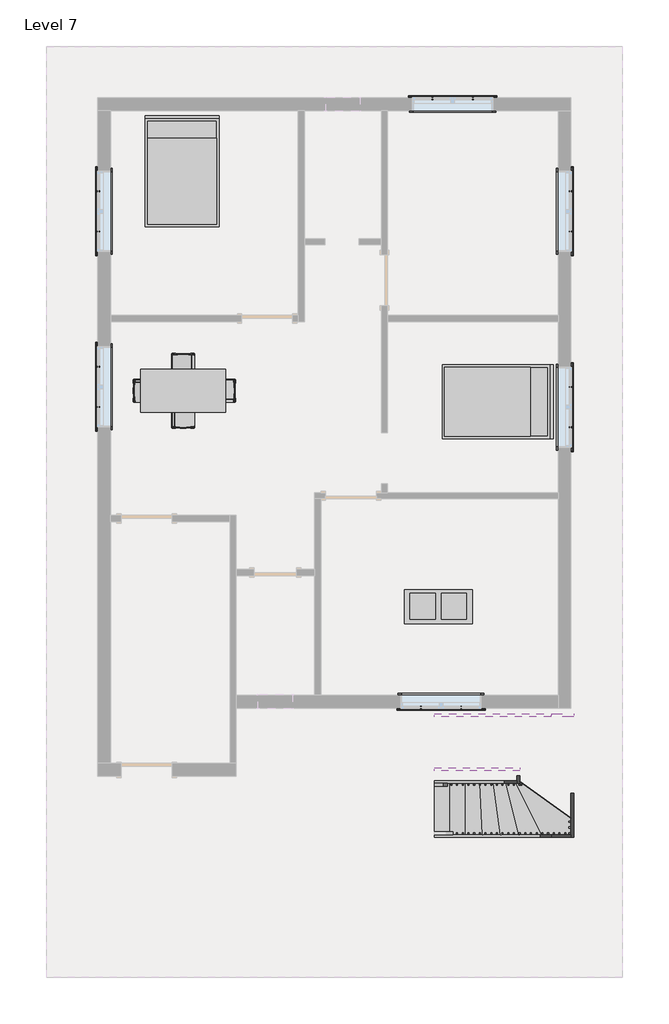
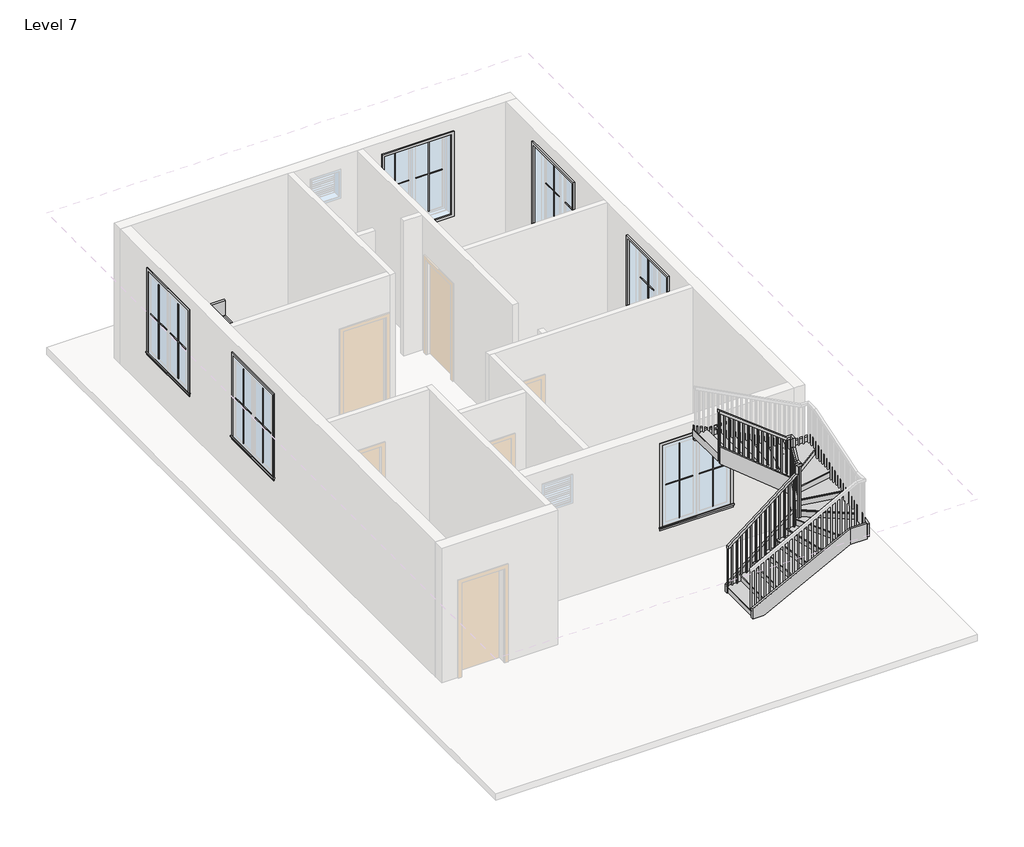
# One storey, part 3 of 3: 25 proxies, 8 members, 3 furniture elements, 1 railing, 1 stair flight.
"""IFC4 building model written with IfcOpenShell, lengths in millimetres."""

from ifc_helpers import new_model, si_unit, frame, origin, place, context, project, spatial, polyline, outline, extrude, faceted_brep, transform, mapped, element, save
from components import muntin_pattern_2x2_muntin_pattern_2x2_bff912c5, muntin_pattern_2x2_muntin_pattern_2x2_c2194282, trim_window_exterior_flat_with_sill_e04b3088, trim_window_interior_flat_picture_frame_2a7685fe, coffee_table_with_brass_mullions_11320_coffee_table_with_5962bef7, bed_17739_bed_17739_15c61121, dining_table_w_chairs_11374_0cdfc61b, stair_flight_09daeeff

model = new_model("IFC4")

# Units and contexts
model_context = context("Model", 3, world=origin())
ifc_project = project(units=[si_unit("LENGTHUNIT", "METRE", prefix="MILLI")], contexts=[model_context])

# Site, building, storey
site = spatial("IfcSite", under=ifc_project)
building = spatial("IfcBuilding", under=site)
storey = spatial("IfcBuildingStorey", under=building, Name="Level 7", Elevation=16002.0)

# Proxies
placement = place(None, origin())
muntin_pattern_2x2_muntin_pattern_2x2_shape = muntin_pattern_2x2_muntin_pattern_2x2_bff912c5(model_context)
element("IfcBuildingElementProxy", 1, Name="Muntin Pattern_2x2 : Muntin Pattern_2x2", ObjectType="Muntin Pattern_2x2 : Muntin Pattern_2x2", at=placement, inside=storey, context=model_context, shape_type="MappedRepresentation", body=[
    mapped(muntin_pattern_2x2_muntin_pattern_2x2_shape, transform((2964.3605034, 427.8534591, 16986.25), x_axis=(0.0, -1.0, 0.0), y_axis=(1.0, 0.0, 0.0), z_axis=(0.0, 0.0, 1.0))),
])
element("IfcBuildingElementProxy", 2, Name="Muntin Pattern_2x2 : Muntin Pattern_2x2", ObjectType="Muntin Pattern_2x2 : Muntin Pattern_2x2", at=placement, inside=storey, context=model_context, shape_type="MappedRepresentation", body=[
    mapped(muntin_pattern_2x2_muntin_pattern_2x2_shape, transform((2964.3605034, 3923.5284591, 16986.25), x_axis=(0.0, -1.0, 0.0), y_axis=(1.0, 0.0, 0.0), z_axis=(0.0, 0.0, 1.0))),
])
element("IfcBuildingElementProxy", 3, Name="Muntin Pattern_2x2 : Muntin Pattern_2x2", ObjectType="Muntin Pattern_2x2 : Muntin Pattern_2x2", at=placement, inside=storey, context=model_context, shape_type="MappedRepresentation", body=[
    mapped(muntin_pattern_2x2_muntin_pattern_2x2_shape, transform((498.9730034, 5582.4659591, 16986.25), x_axis=(1.0, 0.0, 0.0), y_axis=(0.0, 1.0, 0.0), z_axis=(0.0, 0.0, 1.0))),
])
element("IfcBuildingElementProxy", 4, Name="Muntin Pattern_2x2 : Muntin Pattern_2x2", ObjectType="Muntin Pattern_2x2 : Muntin Pattern_2x2", at=placement, inside=storey, context=model_context, shape_type="MappedRepresentation", body=[
    mapped(muntin_pattern_2x2_muntin_pattern_2x2_shape, transform((-5474.7894966, 3202.8034591, 16986.25), x_axis=(0.0, 1.0, 0.0), y_axis=(-1.0, 0.0, 0.0), z_axis=(0.0, 0.0, 1.0))),
])
element("IfcBuildingElementProxy", 5, Name="Muntin Pattern_2x2 : Muntin Pattern_2x2", ObjectType="Muntin Pattern_2x2 : Muntin Pattern_2x2", at=placement, inside=storey, context=model_context, shape_type="MappedRepresentation", body=[
    mapped(muntin_pattern_2x2_muntin_pattern_2x2_shape, transform((-5474.7894966, 69.0784591, 16986.25), x_axis=(0.0, 1.0, 0.0), y_axis=(-1.0, 0.0, 0.0), z_axis=(0.0, 0.0, 1.0))),
])
element("IfcBuildingElementProxy", 6, Name="Muntin Pattern_2x2 : Muntin Pattern_2x2", ObjectType="Muntin Pattern_2x2 : Muntin Pattern_2x2", at=placement, inside=storey, context=model_context, shape_type="MappedRepresentation", body=[
    mapped(muntin_pattern_2x2_muntin_pattern_2x2_shape, transform((1013.3230034, -5295.0840409, 16986.25), x_axis=(-1.0, 0.0, 0.0), y_axis=(0.0, -1.0, 0.0), z_axis=(0.0, 0.0, 1.0))),
])
muntin_pattern_2x2_muntin_pattern_2x2_2_shape = muntin_pattern_2x2_muntin_pattern_2x2_c2194282(model_context)
element("IfcBuildingElementProxy", 7, Name="Muntin Pattern_2x2 : Muntin Pattern_2x2", ObjectType="Muntin Pattern_2x2 : Muntin Pattern_2x2", at=placement, inside=storey, context=model_context, shape_type="MappedRepresentation", body=[
    mapped(muntin_pattern_2x2_muntin_pattern_2x2_2_shape, transform((2964.3605034, -292.8715409, 16986.25), x_axis=(0.0, 1.0, 0.0), y_axis=(-1.0, 0.0, 0.0), z_axis=(0.0, 0.0, 1.0))),
])
element("IfcBuildingElementProxy", 8, Name="Muntin Pattern_2x2 : Muntin Pattern_2x2", ObjectType="Muntin Pattern_2x2 : Muntin Pattern_2x2", at=placement, inside=storey, context=model_context, shape_type="MappedRepresentation", body=[
    mapped(muntin_pattern_2x2_muntin_pattern_2x2_2_shape, transform((2964.3605034, 3202.8034591, 16986.25), x_axis=(0.0, 1.0, 0.0), y_axis=(-1.0, 0.0, 0.0), z_axis=(0.0, 0.0, 1.0))),
])
element("IfcBuildingElementProxy", 9, Name="Muntin Pattern_2x2 : Muntin Pattern_2x2", ObjectType="Muntin Pattern_2x2 : Muntin Pattern_2x2", at=placement, inside=storey, context=model_context, shape_type="MappedRepresentation", body=[
    mapped(muntin_pattern_2x2_muntin_pattern_2x2_2_shape, transform((1219.6980034, 5582.4659591, 16986.25), x_axis=(-1.0, 0.0, 0.0), y_axis=(0.0, -1.0, 0.0), z_axis=(0.0, 0.0, 1.0))),
])
element("IfcBuildingElementProxy", 10, Name="Muntin Pattern_2x2 : Muntin Pattern_2x2", ObjectType="Muntin Pattern_2x2 : Muntin Pattern_2x2", at=placement, inside=storey, context=model_context, shape_type="MappedRepresentation", body=[
    mapped(muntin_pattern_2x2_muntin_pattern_2x2_2_shape, transform((-5474.7894966, 3923.5284591, 16986.25), x_axis=(0.0, -1.0, 0.0), y_axis=(1.0, 0.0, 0.0), z_axis=(0.0, 0.0, 1.0))),
])
element("IfcBuildingElementProxy", 11, Name="Muntin Pattern_2x2 : Muntin Pattern_2x2", ObjectType="Muntin Pattern_2x2 : Muntin Pattern_2x2", at=placement, inside=storey, context=model_context, shape_type="MappedRepresentation", body=[
    mapped(muntin_pattern_2x2_muntin_pattern_2x2_2_shape, transform((-5474.7894966, 789.8034591, 16986.25), x_axis=(0.0, -1.0, 0.0), y_axis=(1.0, 0.0, 0.0), z_axis=(0.0, 0.0, 1.0))),
])
element("IfcBuildingElementProxy", 12, Name="Muntin Pattern_2x2 : Muntin Pattern_2x2", ObjectType="Muntin Pattern_2x2 : Muntin Pattern_2x2", at=placement, inside=storey, context=model_context, shape_type="MappedRepresentation", body=[
    mapped(muntin_pattern_2x2_muntin_pattern_2x2_2_shape, transform((292.5980034, -5295.0840409, 16986.25), x_axis=(1.0, 0.0, 0.0), y_axis=(0.0, 1.0, 0.0), z_axis=(0.0, 0.0, 1.0))),
])
trim_window_exterior_flat_with_sill_shape = trim_window_exterior_flat_with_sill_e04b3088(model_context)
element("IfcBuildingElementProxy", 13, Name="Trim-Window-Exterior-Flat : with Sill", ObjectType="Trim-Window-Exterior-Flat : with Sill", at=placement, inside=storey, context=model_context, shape_type="MappedRepresentation", body=[
    mapped(trim_window_exterior_flat_with_sill_shape, transform((2973.8855034, 67.4909591, 18745.2), x_axis=(0.0, 1.0, 0.0), y_axis=(0.0, 0.0, 1.0), z_axis=(1.0, 0.0, 0.0))),
])
element("IfcBuildingElementProxy", 14, Name="Trim-Window-Exterior-Flat : with Sill", ObjectType="Trim-Window-Exterior-Flat : with Sill", at=placement, inside=storey, context=model_context, shape_type="MappedRepresentation", body=[
    mapped(trim_window_exterior_flat_with_sill_shape, transform((2973.8855034, 3563.1659591, 18745.2), x_axis=(0.0, 1.0, 0.0), y_axis=(0.0, 0.0, 1.0), z_axis=(1.0, 0.0, 0.0))),
])
element("IfcBuildingElementProxy", 15, Name="Trim-Window-Exterior-Flat : with Sill", ObjectType="Trim-Window-Exterior-Flat : with Sill", at=placement, inside=storey, context=model_context, shape_type="MappedRepresentation", body=[
    mapped(trim_window_exterior_flat_with_sill_shape, transform((859.3355034, 5591.9909591, 18745.2), x_axis=(-1.0, 0.0, 0.0), y_axis=(0.0, 0.0, 1.0), z_axis=(0.0, 1.0, 0.0))),
])
element("IfcBuildingElementProxy", 16, Name="Trim-Window-Exterior-Flat : with Sill", ObjectType="Trim-Window-Exterior-Flat : with Sill", at=placement, inside=storey, context=model_context, shape_type="MappedRepresentation", body=[
    mapped(trim_window_exterior_flat_with_sill_shape, transform((-5484.3144966, 3563.1659591, 18745.2), x_axis=(0.0, -1.0, 0.0), y_axis=(0.0, 0.0, 1.0), z_axis=(-1.0, 0.0, 0.0))),
])
element("IfcBuildingElementProxy", 17, Name="Trim-Window-Exterior-Flat : with Sill", ObjectType="Trim-Window-Exterior-Flat : with Sill", at=placement, inside=storey, context=model_context, shape_type="MappedRepresentation", body=[
    mapped(trim_window_exterior_flat_with_sill_shape, transform((-5484.3144966, 429.4409591, 18745.2), x_axis=(0.0, -1.0, 0.0), y_axis=(0.0, 0.0, 1.0), z_axis=(-1.0, 0.0, 0.0))),
])
element("IfcBuildingElementProxy", 18, Name="Trim-Window-Exterior-Flat : with Sill", ObjectType="Trim-Window-Exterior-Flat : with Sill", at=placement, inside=storey, context=model_context, shape_type="MappedRepresentation", body=[
    mapped(trim_window_exterior_flat_with_sill_shape, transform((652.9605034, -5304.6090409, 18745.2), x_axis=(1.0, 0.0, 0.0), y_axis=(0.0, 0.0, 1.0), z_axis=(0.0, -1.0, 0.0))),
])
trim_window_interior_flat_picture_frame_shape = trim_window_interior_flat_picture_frame_2a7685fe(model_context)
element("IfcBuildingElementProxy", 19, Name="Trim-Window-Interior-Flat : Picture Frame", ObjectType="Trim-Window-Interior-Flat : Picture Frame", at=placement, inside=storey, context=model_context, shape_type="MappedRepresentation", body=[
    mapped(trim_window_interior_flat_picture_frame_shape, transform((2745.2855034, 67.4909591, 18745.2), x_axis=(0.0, -1.0, 0.0), y_axis=(0.0, 0.0, 1.0), z_axis=(-1.0, 0.0, 0.0))),
])
element("IfcBuildingElementProxy", 20, Name="Trim-Window-Interior-Flat : Picture Frame", ObjectType="Trim-Window-Interior-Flat : Picture Frame", at=placement, inside=storey, context=model_context, shape_type="MappedRepresentation", body=[
    mapped(trim_window_interior_flat_picture_frame_shape, transform((2745.2855034, 3563.1659591, 18745.2), x_axis=(0.0, -1.0, 0.0), y_axis=(0.0, 0.0, 1.0), z_axis=(-1.0, 0.0, 0.0))),
])
element("IfcBuildingElementProxy", 21, Name="Trim-Window-Interior-Flat : Picture Frame", ObjectType="Trim-Window-Interior-Flat : Picture Frame", at=placement, inside=storey, context=model_context, shape_type="MappedRepresentation", body=[
    mapped(trim_window_interior_flat_picture_frame_shape, transform((859.3355034, 5363.3909591, 18745.2), x_axis=(1.0, 0.0, 0.0), y_axis=(0.0, 0.0, 1.0), z_axis=(0.0, -1.0, 0.0))),
])
element("IfcBuildingElementProxy", 22, Name="Trim-Window-Interior-Flat : Picture Frame", ObjectType="Trim-Window-Interior-Flat : Picture Frame", at=placement, inside=storey, context=model_context, shape_type="MappedRepresentation", body=[
    mapped(trim_window_interior_flat_picture_frame_shape, transform((-5255.7144966, 3563.1659591, 18745.2), x_axis=(0.0, 1.0, 0.0), y_axis=(0.0, 0.0, 1.0), z_axis=(1.0, 0.0, 0.0))),
])
element("IfcBuildingElementProxy", 23, Name="Trim-Window-Interior-Flat : Picture Frame", ObjectType="Trim-Window-Interior-Flat : Picture Frame", at=placement, inside=storey, context=model_context, shape_type="MappedRepresentation", body=[
    mapped(trim_window_interior_flat_picture_frame_shape, transform((-5255.7144966, 429.4409591, 18745.2), x_axis=(0.0, 1.0, 0.0), y_axis=(0.0, 0.0, 1.0), z_axis=(1.0, 0.0, 0.0))),
])
element("IfcBuildingElementProxy", 24, Name="Trim-Window-Interior-Flat : Picture Frame", ObjectType="Trim-Window-Interior-Flat : Picture Frame", at=placement, inside=storey, context=model_context, shape_type="MappedRepresentation", body=[
    mapped(trim_window_interior_flat_picture_frame_shape, transform((652.9605034, -5076.0090409, 18745.2), x_axis=(-1.0, 0.0, 0.0), y_axis=(0.0, 0.0, 1.0), z_axis=(0.0, 1.0, 0.0))),
])
coffee_table_with_brass_mullions_11320_coffee_table_with_shape = coffee_table_with_brass_mullions_11320_coffee_table_with_5962bef7(model_context)
element("IfcBuildingElementProxy", 25, Name="coffee_table_with_brass_mullions_11320 : coffee_table_with_brass_mullions_11320", ObjectType="coffee_table_with_brass_mullions_11320 : coffee_table_with_brass_mullions_11320", at=placement, inside=storey, context=model_context, shape_type="MappedRepresentation", body=[
    mapped(coffee_table_with_brass_mullions_11320_coffee_table_with_shape, transform((1240.0943553, -3926.0808329, 16002.0), x_axis=(1.0, 0.0, 0.0), y_axis=(0.0, 1.0, 0.0), z_axis=(0.0, 0.0, 1.0))),
])

# Furniture
bed_17739_bed_17739_shape = bed_17739_bed_17739_15c61121(model_context)
element("IfcFurniture", 26, ObjectType="Bed_17739 : Bed_17739", at=placement, inside=storey, context=model_context, shape_type="MappedRepresentation", body=[
    mapped(bed_17739_bed_17739_shape, transform((-3979.3644966, 4258.4909591, 16002.0), x_axis=(1.0, 0.0, 0.0), y_axis=(0.0, 1.0, 0.0), z_axis=(0.0, 0.0, 1.0))),
])
element("IfcFurniture", 27, ObjectType="Bed_17739 : Bed_17739", at=placement, inside=storey, context=model_context, shape_type="MappedRepresentation", body=[
    mapped(bed_17739_bed_17739_shape, transform((1640.3855034, 162.7409591, 16002.0), x_axis=(0.0, -1.0, 0.0), y_axis=(1.0, 0.0, 0.0), z_axis=(0.0, 0.0, 1.0))),
])
dining_table_w_chairs_11374_shape = dining_table_w_chairs_11374_0cdfc61b(model_context)
element("IfcFurniture", 28, ObjectType="Dining_Table_w_Chairs_11374", at=placement, inside=storey, context=model_context, shape_type="MappedRepresentation", body=[
    mapped(dining_table_w_chairs_11374_shape, transform((-3975.2132663, 265.1952874, 16002.0), x_axis=(1.0, 0.0, 0.0), y_axis=(0.0, 1.0, 0.0), z_axis=(0.0, 0.0, 1.0))),
])

# Members
element("IfcMember", 29, ObjectType="Stringer - 2\" Width", at=placement, inside=storey, context=model_context, shape_type="SweptSolid", body=[
    extrude(outline(polyline([(16178.1764461, 531.7538115), (16002.0, 531.7538115), (16002.0, 798.0154561), (16989.1410923, 2008.6855034), (17382.418648, 2008.6855034), (16178.1764461, 531.7538115)])), frame((0.0, -6650.8090409, 0.0), z_axis=(0.0, 1.0, 0.0), x_axis=(0.0, 0.0, 1.0)), (0.0, 0.0, 1.0), 50.8),
])
element("IfcMember", 30, ObjectType="Stringer - 2\" Width", at=placement, inside=storey, context=model_context, shape_type="SweptSolid", body=[
    extrude(outline(polyline([(-6650.8090409, 17030.5617647), (-6650.8090409, 17575.2682978), (-6444.1719234, 17928.1409689), (-6422.2090409, 17928.1409689), (-6422.2090409, 17362.465107), (-6616.5668235, 17030.5617647), (-6650.8090409, 17030.5617647)])), frame((2008.6855034, 0.0, 0.0), z_axis=(1.0, 0.0, 0.0), x_axis=(0.0, 1.0, 0.0)), (0.0, 0.0, 1.0), 50.8),
])
element("IfcMember", 31, ObjectType="Stringer - 2\" Width", at=placement, inside=storey, context=model_context, shape_type="SweptSolid", body=[
    extrude(outline(polyline([(17534.8634131, 2059.4855034), (17928.1409689, 2059.4855034), (19173.8038432, 531.7538115), (18780.5262875, 531.7538115), (17534.8634131, 2059.4855034)])), frame((0.0, -6422.2090409, 0.0), z_axis=(0.0, 1.0, 0.0), x_axis=(0.0, 0.0, 1.0)), (0.0, 0.0, 1.0), 50.8),
])
element("IfcMember", 32, ObjectType="Stringer - 2\" Width", at=placement, inside=storey, context=model_context, shape_type="SweptSolid", body=[
    extrude(outline(polyline([(16231.639954, 531.7538115), (16002.0, 531.7538115), (16002.0, 751.5161291), (16964.500629, 2619.1710032), (17307.3956453, 2619.1710032), (16231.639954, 531.7538115)])), frame((0.0, -7616.0090409, 0.0), z_axis=(0.0, 1.0, 0.0), x_axis=(0.0, 0.0, 1.0)), (0.0, 0.0, 1.0), 50.8),
])
element("IfcMember", 33, ObjectType="Stringer - 2\" Width", at=placement, inside=storey, context=model_context, shape_type="SweptSolid", body=[
    extrude(outline(polyline([(2619.1710032, -7616.0090409), (2619.1710032, -7565.2090409), (2973.8855034, -7565.2090409), (2973.8855034, -7616.0090409), (2619.1710032, -7616.0090409)])), frame((0.0, 0.0, 16964.500629), z_axis=(0.0, 0.0, 1.0), x_axis=(1.0, 0.0, 0.0)), (0.0, 0.0, 1.0), 342.8950162),
])
element("IfcMember", 34, ObjectType="Stringer - 2\" Width", at=placement, inside=storey, context=model_context, shape_type="SweptSolid", body=[
    extrude(outline(polyline([(-7616.0090409, 17002.5956453), (-7616.0090409, 17291.0952212), (-5493.9891581, 17971.9972697), (-5457.0090409, 17971.9972697), (-5457.0090409, 17640.9682298), (-7446.4865579, 17002.5956453), (-7616.0090409, 17002.5956453)])), frame((2973.8855034, 0.0, 0.0), z_axis=(1.0, 0.0, 0.0), x_axis=(0.0, 1.0, 0.0)), (0.0, 0.0, 1.0), 50.8),
])
element("IfcMember", 35, ObjectType="Stringer - 2\" Width", at=placement, inside=storey, context=model_context, shape_type="SweptSolid", body=[
    extrude(outline(polyline([(3024.6855034, -5406.2090409), (3024.6855034, -5457.0090409), (2619.1710032, -5457.0090409), (2619.1710032, -5406.2090409), (3024.6855034, -5406.2090409)])), frame((0.0, 0.0, 17651.8904473), z_axis=(0.0, 0.0, 1.0), x_axis=(1.0, 0.0, 0.0)), (0.0, 0.0, 1.0), 320.1068224),
])
element("IfcMember", 36, ObjectType="Stringer - 2\" Width", at=placement, inside=storey, context=model_context, shape_type="SweptSolid", body=[
    extrude(outline(polyline([(17651.8904473, 2619.1710032), (17971.9972697, 2619.1710032), (19047.7529609, 531.7538115), (18727.6461385, 531.7538115), (17651.8904473, 2619.1710032)])), frame((0.0, -5457.0090409, 0.0), z_axis=(0.0, 1.0, 0.0), x_axis=(0.0, 0.0, 1.0)), (0.0, 0.0, 1.0), 50.8),
])

# Railing
element("IfcRailing", 37, ObjectType="Handrail - Rectangular", at=placement, inside=storey, context=model_context, shape_type="SolidModel", body=[
    faceted_brep([(531.7538115, -6650.8090409, 17085.7333333), (531.7538115, -6650.8090409, 17021.4000346), (531.7538115, -6701.6090409, 17021.4000346), (531.7538115, -6701.6090409, 17085.7333333), (1983.2855034, -6650.8090409, 18213.6191036), (2034.0855034, -6650.8090409, 18188.7590024), (2034.0855034, -6701.6090409, 18188.7590024), (1983.2855034, -6701.6090409, 18213.6191036), (2059.4855034, -6545.487707, 18365.8281882), (2059.4855034, -6574.6090409, 18416.6281882), (2059.4855034, -6447.6090409, 18633.5051451), (2059.4855034, -6396.8090409, 18619.7256424), (2110.2855034, -6545.487707, 18365.8281882), (2110.2855034, -6396.8090409, 18619.7256424), (2110.2855034, -6574.6090409, 18416.6281882), (2110.2855034, -6447.6090409, 18633.5051451), (531.7538115, -6371.4090409, 19964.4), (531.7538115, -6320.6090409, 19964.4), (531.7538115, -6320.6090409, 19900.0667013), (531.7538115, -6371.4090409, 19900.0667013), (1965.8688354, -6371.4090409, 18785.7142297), (1983.2855034, -6371.4090409, 18836.5142297), (1965.8688354, -6320.6090409, 18785.7142297), (1983.2855034, -6320.6090409, 18836.5142297), (1983.2855034, -6650.8090409, 18416.6281882), (2034.0855034, -6650.8090409, 18365.8281882), (2034.0855034, -6701.6090409, 18365.8281882), (1983.2855034, -6701.6090409, 18416.6281882), (2059.4855034, -6650.8090409, 18416.6281882), (2059.4855034, -6650.8090409, 18365.8281882), (2110.2855034, -6701.6090409, 18365.8281882), (2110.2855034, -6701.6090409, 18416.6281882), (2059.4855034, -6447.6090409, 18836.5142297), (2059.4855034, -6396.8090409, 18785.7142297), (2110.2855034, -6396.8090409, 18785.7142297), (2110.2855034, -6447.6090409, 18836.5142297), (2059.4855034, -6371.4090409, 18836.5142297), (2059.4855034, -6371.4090409, 18785.7142297), (2110.2855034, -6320.6090409, 18785.7142297), (2110.2855034, -6320.6090409, 18836.5142297)], [[[0, 1, 2, 3]], [[1, 0, 4, 5]], [[2, 1, 5, 6]], [[3, 2, 6, 7]], [[0, 3, 7, 4]], [[8, 9, 10, 11]], [[12, 8, 11, 13]], [[14, 12, 13, 15]], [[9, 14, 15, 10]], [[16, 17, 18, 19]], [[20, 21, 16, 19]], [[22, 20, 19, 18]], [[23, 22, 18, 17]], [[21, 23, 17, 16]], [[5, 4, 24, 25]], [[6, 5, 25, 26]], [[7, 6, 26, 27]], [[4, 7, 27, 24]], [[25, 24, 28, 29]], [[26, 25, 29, 30]], [[27, 26, 30, 31]], [[24, 27, 31, 28]], [[29, 28, 9, 8]], [[30, 29, 8, 12]], [[31, 30, 12, 14]], [[28, 31, 14, 9]], [[11, 10, 32, 33]], [[13, 11, 33, 34]], [[15, 13, 34, 35]], [[10, 15, 35, 32]], [[33, 32, 36, 37]], [[34, 33, 37, 38]], [[35, 34, 38, 39]], [[32, 35, 39, 36]], [[37, 36, 21, 20]], [[38, 37, 20, 22]], [[39, 38, 22, 23]], [[36, 39, 23, 21]]]),
    extrude(outline(polyline([(19884.8316852, 551.3605034), (18880.6666667, 551.3605034), (18880.6666667, 570.4105034), (19870.0292361, 570.4105034), (19884.8316852, 551.3605034)])), frame((0.0, -6355.5340409, 0.0), z_axis=(0.0, 1.0, 0.0), x_axis=(0.0, 0.0, 1.0)), (0.0, 0.0, 1.0), 19.05),
    extrude(outline(polyline([(19805.8852902, 652.9605034), (18880.6666667, 652.9605034), (18880.6666667, 672.0105034), (19791.0828411, 672.0105034), (19805.8852902, 652.9605034)])), frame((0.0, -6355.5340409, 0.0), z_axis=(0.0, 1.0, 0.0), x_axis=(0.0, 0.0, 1.0)), (0.0, 0.0, 1.0), 19.05),
    extrude(outline(polyline([(19726.9388952, 754.5605034), (18880.6666667, 754.5605034), (18880.6666667, 773.6105034), (19712.1364462, 773.6105034), (19726.9388952, 754.5605034)])), frame((0.0, -6355.5340409, 0.0), z_axis=(0.0, 1.0, 0.0), x_axis=(0.0, 0.0, 1.0)), (0.0, 0.0, 1.0), 19.05),
    extrude(outline(polyline([(19647.9925003, 856.1605034), (18711.3333333, 856.1605034), (18711.3333333, 875.2105034), (19633.1900512, 875.2105034), (19647.9925003, 856.1605034)])), frame((0.0, -6355.5340409, 0.0), z_axis=(0.0, 1.0, 0.0), x_axis=(0.0, 0.0, 1.0)), (0.0, 0.0, 1.0), 19.05),
    extrude(outline(polyline([(19569.0461053, 957.7605034), (18711.3333333, 957.7605034), (18711.3333333, 976.8105034), (19554.2436562, 976.8105034), (19569.0461053, 957.7605034)])), frame((0.0, -6355.5340409, 0.0), z_axis=(0.0, 1.0, 0.0), x_axis=(0.0, 0.0, 1.0)), (0.0, 0.0, 1.0), 19.05),
    extrude(outline(polyline([(19490.0997103, 1059.3605034), (18711.3333333, 1059.3605034), (18711.3333333, 1078.4105034), (19475.2972613, 1078.4105034), (19490.0997103, 1059.3605034)])), frame((0.0, -6355.5340409, 0.0), z_axis=(0.0, 1.0, 0.0), x_axis=(0.0, 0.0, 1.0)), (0.0, 0.0, 1.0), 19.05),
    extrude(outline(polyline([(19411.1533154, 1160.9605034), (18542.0, 1160.9605034), (18542.0, 1180.0105034), (19396.3508663, 1180.0105034), (19411.1533154, 1160.9605034)])), frame((0.0, -6355.5340409, 0.0), z_axis=(0.0, 1.0, 0.0), x_axis=(0.0, 0.0, 1.0)), (0.0, 0.0, 1.0), 19.05),
    extrude(outline(polyline([(19332.2069204, 1262.5605034), (18542.0, 1262.5605034), (18542.0, 1281.6105034), (19317.4044713, 1281.6105034), (19332.2069204, 1262.5605034)])), frame((0.0, -6355.5340409, 0.0), z_axis=(0.0, 1.0, 0.0), x_axis=(0.0, 0.0, 1.0)), (0.0, 0.0, 1.0), 19.05),
    extrude(outline(polyline([(19253.2605254, 1364.1605034), (18372.6666667, 1364.1605034), (18372.6666667, 1383.2105034), (19238.4580764, 1383.2105034), (19253.2605254, 1364.1605034)])), frame((0.0, -6355.5340409, 0.0), z_axis=(0.0, 1.0, 0.0), x_axis=(0.0, 0.0, 1.0)), (0.0, 0.0, 1.0), 19.05),
    extrude(outline(polyline([(19174.3141304, 1465.7605034), (18372.6666667, 1465.7605034), (18372.6666667, 1484.8105034), (19159.5116814, 1484.8105034), (19174.3141304, 1465.7605034)])), frame((0.0, -6355.5340409, 0.0), z_axis=(0.0, 1.0, 0.0), x_axis=(0.0, 0.0, 1.0)), (0.0, 0.0, 1.0), 19.05),
    extrude(outline(polyline([(19095.3677355, 1567.3605034), (18372.6666667, 1567.3605034), (18372.6666667, 1586.4105034), (19080.5652864, 1586.4105034), (19095.3677355, 1567.3605034)])), frame((0.0, -6355.5340409, 0.0), z_axis=(0.0, 1.0, 0.0), x_axis=(0.0, 0.0, 1.0)), (0.0, 0.0, 1.0), 19.05),
    extrude(outline(polyline([(19016.4213405, 1668.9605034), (18203.3333333, 1668.9605034), (18203.3333333, 1688.0105034), (19001.6188914, 1688.0105034), (19016.4213405, 1668.9605034)])), frame((0.0, -6355.5340409, 0.0), z_axis=(0.0, 1.0, 0.0), x_axis=(0.0, 0.0, 1.0)), (0.0, 0.0, 1.0), 19.05),
    extrude(outline(polyline([(18937.4749455, 1770.5605034), (18203.3333333, 1770.5605034), (18203.3333333, 1789.6105034), (18922.6724965, 1789.6105034), (18937.4749455, 1770.5605034)])), frame((0.0, -6355.5340409, 0.0), z_axis=(0.0, 1.0, 0.0), x_axis=(0.0, 0.0, 1.0)), (0.0, 0.0, 1.0), 19.05),
    extrude(outline(polyline([(18858.5285506, 1872.1605034), (18034.0, 1872.1605034), (18034.0, 1891.2105034), (18843.7261015, 1891.2105034), (18858.5285506, 1872.1605034)])), frame((0.0, -6355.5340409, 0.0), z_axis=(0.0, 1.0, 0.0), x_axis=(0.0, 0.0, 1.0)), (0.0, 0.0, 1.0), 19.05),
    extrude(outline(polyline([(18779.5821556, 1973.7605034), (18034.0, 1973.7605034), (18034.0, 1992.8105034), (18764.7797065, 1992.8105034), (18779.5821556, 1973.7605034)])), frame((0.0, -6355.5340409, 0.0), z_axis=(0.0, 1.0, 0.0), x_axis=(0.0, 0.0, 1.0)), (0.0, 0.0, 1.0), 19.05),
    extrude(outline(polyline([(2075.3605034, -6380.9340409), (2075.3605034, -6361.8840409), (2094.4105034, -6361.8840409), (2094.4105034, -6380.9340409), (2075.3605034, -6380.9340409)])), frame((0.0, 0.0, 17695.3333333), z_axis=(0.0, 0.0, 1.0), x_axis=(1.0, 0.0, 0.0)), (0.0, 0.0, 1.0), 1090.3808964),
    extrude(outline(polyline([(-6463.4840409, 18505.86524), (-6463.4840409, 17526.0), (-6482.5340409, 17526.0), (-6482.5340409, 18473.3336964), (-6463.4840409, 18505.86524)])), frame((2075.3605034, 0.0, 0.0), z_axis=(1.0, 0.0, 0.0), x_axis=(0.0, 1.0, 0.0)), (0.0, 0.0, 1.0), 19.05),
    extrude(outline(polyline([(-6565.0840409, 18332.3636744), (-6565.0840409, 17356.6666667), (-6584.1340409, 17356.6666667), (-6584.1340409, 18299.8321309), (-6565.0840409, 18332.3636744)])), frame((2075.3605034, 0.0, 0.0), z_axis=(1.0, 0.0, 0.0), x_axis=(0.0, 1.0, 0.0)), (0.0, 0.0, 1.0), 19.05),
    extrude(outline(polyline([(2046.2288115, -6666.6840409), (2065.2788115, -6666.6840409), (2065.2788115, -6685.7340409), (2046.2288115, -6685.7340409), (2046.2288115, -6666.6840409)])), frame((0.0, 0.0, 17187.3333333), z_axis=(0.0, 0.0, 1.0), x_axis=(1.0, 0.0, 0.0)), (0.0, 0.0, 1.0), 1178.4948549),
    extrude(outline(polyline([(18119.2483397, 1944.6288115), (17018.0, 1944.6288115), (17018.0, 1963.6788115), (18134.0507888, 1963.6788115), (18119.2483397, 1944.6288115)])), frame((0.0, -6685.7340409, 0.0), z_axis=(0.0, 1.0, 0.0), x_axis=(0.0, 0.0, 1.0)), (0.0, 0.0, 1.0), 19.05),
    extrude(outline(polyline([(18040.3019447, 1843.0288115), (17018.0, 1843.0288115), (17018.0, 1862.0788115), (18055.1043938, 1862.0788115), (18040.3019447, 1843.0288115)])), frame((0.0, -6685.7340409, 0.0), z_axis=(0.0, 1.0, 0.0), x_axis=(0.0, 0.0, 1.0)), (0.0, 0.0, 1.0), 19.05),
    extrude(outline(polyline([(17961.3555498, 1741.4288115), (16848.6666667, 1741.4288115), (16848.6666667, 1760.4788115), (17976.1579988, 1760.4788115), (17961.3555498, 1741.4288115)])), frame((0.0, -6685.7340409, 0.0), z_axis=(0.0, 1.0, 0.0), x_axis=(0.0, 0.0, 1.0)), (0.0, 0.0, 1.0), 19.05),
    extrude(outline(polyline([(17882.4091548, 1639.8288115), (16848.6666667, 1639.8288115), (16848.6666667, 1658.8788115), (17897.2116039, 1658.8788115), (17882.4091548, 1639.8288115)])), frame((0.0, -6685.7340409, 0.0), z_axis=(0.0, 1.0, 0.0), x_axis=(0.0, 0.0, 1.0)), (0.0, 0.0, 1.0), 19.05),
    extrude(outline(polyline([(17803.4627598, 1538.2288115), (16679.3333333, 1538.2288115), (16679.3333333, 1557.2788115), (17818.2652089, 1557.2788115), (17803.4627598, 1538.2288115)])), frame((0.0, -6685.7340409, 0.0), z_axis=(0.0, 1.0, 0.0), x_axis=(0.0, 0.0, 1.0)), (0.0, 0.0, 1.0), 19.05),
    extrude(outline(polyline([(17724.5163649, 1436.6288115), (16679.3333333, 1436.6288115), (16679.3333333, 1455.6788115), (17739.3188139, 1455.6788115), (17724.5163649, 1436.6288115)])), frame((0.0, -6685.7340409, 0.0), z_axis=(0.0, 1.0, 0.0), x_axis=(0.0, 0.0, 1.0)), (0.0, 0.0, 1.0), 19.05),
    extrude(outline(polyline([(17645.5699699, 1335.0288115), (16510.0, 1335.0288115), (16510.0, 1354.0788115), (17660.3724189, 1354.0788115), (17645.5699699, 1335.0288115)])), frame((0.0, -6685.7340409, 0.0), z_axis=(0.0, 1.0, 0.0), x_axis=(0.0, 0.0, 1.0)), (0.0, 0.0, 1.0), 19.05),
    extrude(outline(polyline([(17566.6235749, 1233.4288115), (16510.0, 1233.4288115), (16510.0, 1252.4788115), (17581.426024, 1252.4788115), (17566.6235749, 1233.4288115)])), frame((0.0, -6685.7340409, 0.0), z_axis=(0.0, 1.0, 0.0), x_axis=(0.0, 0.0, 1.0)), (0.0, 0.0, 1.0), 19.05),
    extrude(outline(polyline([(17487.6771799, 1131.8288115), (16510.0, 1131.8288115), (16510.0, 1150.8788115), (17502.479629, 1150.8788115), (17487.6771799, 1131.8288115)])), frame((0.0, -6685.7340409, 0.0), z_axis=(0.0, 1.0, 0.0), x_axis=(0.0, 0.0, 1.0)), (0.0, 0.0, 1.0), 19.05),
    extrude(outline(polyline([(17408.730785, 1030.2288115), (16340.6666667, 1030.2288115), (16340.6666667, 1049.2788115), (17423.533234, 1049.2788115), (17408.730785, 1030.2288115)])), frame((0.0, -6685.7340409, 0.0), z_axis=(0.0, 1.0, 0.0), x_axis=(0.0, 0.0, 1.0)), (0.0, 0.0, 1.0), 19.05),
    extrude(outline(polyline([(17329.78439, 928.6288115), (16340.6666667, 928.6288115), (16340.6666667, 947.6788115), (17344.5868391, 947.6788115), (17329.78439, 928.6288115)])), frame((0.0, -6685.7340409, 0.0), z_axis=(0.0, 1.0, 0.0), x_axis=(0.0, 0.0, 1.0)), (0.0, 0.0, 1.0), 19.05),
    extrude(outline(polyline([(17250.837995, 827.0288115), (16340.6666667, 827.0288115), (16340.6666667, 846.0788115), (17265.6404441, 846.0788115), (17250.837995, 827.0288115)])), frame((0.0, -6685.7340409, 0.0), z_axis=(0.0, 1.0, 0.0), x_axis=(0.0, 0.0, 1.0)), (0.0, 0.0, 1.0), 19.05),
    extrude(outline(polyline([(17171.8916001, 725.4288115), (16171.3333333, 725.4288115), (16171.3333333, 744.4788115), (17186.6940491, 744.4788115), (17171.8916001, 725.4288115)])), frame((0.0, -6685.7340409, 0.0), z_axis=(0.0, 1.0, 0.0), x_axis=(0.0, 0.0, 1.0)), (0.0, 0.0, 1.0), 19.05),
    extrude(outline(polyline([(17092.9452051, 623.8288115), (16171.3333333, 623.8288115), (16171.3333333, 642.8788115), (17107.7476541, 642.8788115), (17092.9452051, 623.8288115)])), frame((0.0, -6685.7340409, 0.0), z_axis=(0.0, 1.0, 0.0), x_axis=(0.0, 0.0, 1.0)), (0.0, 0.0, 1.0), 19.05),
    extrude(outline(polyline([(2075.3605034, -6355.5340409), (2075.3605034, -6336.4840409), (2094.4105034, -6336.4840409), (2094.4105034, -6355.5340409), (2075.3605034, -6355.5340409)])), frame((0.0, 0.0, 17864.6666667), z_axis=(0.0, 0.0, 1.0), x_axis=(1.0, 0.0, 0.0)), (0.0, 0.0, 1.0), 921.0475631),
    extrude(outline(polyline([(2075.3605034, -6666.6840409), (2094.4105034, -6666.6840409), (2094.4105034, -6685.7340409), (2075.3605034, -6685.7340409), (2075.3605034, -6666.6840409)])), frame((0.0, 0.0, 17187.3333333), z_axis=(0.0, 0.0, 1.0), x_axis=(1.0, 0.0, 0.0)), (0.0, 0.0, 1.0), 1178.4948549),
    extrude(outline(polyline([(19900.0667013, 531.7538115), (18880.6666667, 531.7538115), (18880.6666667, 550.8038115), (19885.2642523, 550.8038115), (19900.0667013, 531.7538115)])), frame((0.0, -6355.5340409, 0.0), z_axis=(0.0, 1.0, 0.0), x_axis=(0.0, 0.0, 1.0)), (0.0, 0.0, 1.0), 19.05),
    extrude(outline(polyline([(17021.4000346, 531.7538115), (16171.3333333, 531.7538115), (16171.3333333, 550.8038115), (17036.2024837, 550.8038115), (17021.4000346, 531.7538115)])), frame((0.0, -6685.7340409, 0.0), z_axis=(0.0, 1.0, 0.0), x_axis=(0.0, 0.0, 1.0)), (0.0, 0.0, 1.0), 19.05),
])

# Stair flight
stair_flight_shape = stair_flight_09daeeff(model_context)
element("IfcStairFlight", 38, ObjectType="2\" Tread 1\" Nosing 1/4\" Riser", at=placement, inside=storey, context=model_context, shape_type="MappedRepresentation", body=[
    mapped(stair_flight_shape, transform((0.0, 0.0, 0.0), x_axis=(1.0, 0.0, 0.0), y_axis=(0.0, 1.0, 0.0), z_axis=(0.0, 0.0, 1.0))),
])

save(model, "model.ifc")

# Revit data of these elements
# Type "Muntin Pattern_2x2 : Muntin Pattern_2x2"
#   Width [instance default] = 4' - 0"
#   Thickness = 0' - 0 1/2"
#   Height [instance default] = 4' - 0"
#   Distance = 0' - 0 3/4"
#   Interior Material [instance default] = none
#   Exterior Material [instance default] = none
#   Default Elevation = 0
# Type "Trim-Window-Exterior-Flat : with Sill"
#   Trim Width = 0' - 2 1/4"
#   Trim Thickness_Picture Frame = 0' - 1 1/4"
#   Trim Thickness_with Sill = 0' - 0 3/4"
#   Sill Thickness = 0' - 1 1/4"
#   Opening Width [instance default] = 2' - 0"
#   Opening Height [instance default] = 3' - 0"
#   Default Elevation = 4' - 0"
#   Sill = yes
#   Picture Frame = no
#   Trim Material [instance default] = none
# Type "Trim-Window-Interior-Flat : Picture Frame"
#   Trim Thickness_Picture Frame = 0' - 1 1/4"
#   Trim Width = 0' - 2 1/4"
#   Trim Thickness_with Sill = 0' - 0 3/4"
#   Sill Thickness = 0' - 1 1/4"
#   Opening Width [instance default] = 2' - 0"
#   Opening Height [instance default] = 3' - 0"
#   Default Elevation = 4' - 0"
#   Sill = no
#   Picture Frame = yes
#   Trim Material [instance default] = none
# Type "coffee_table_with_brass_mullions_11320 : coffee_table_with_brass_mullions_11320"
#   Default Elevation = 0
# Type "Bed_17739 : Bed_17739"
#   Default Elevation = 0
# Type "Dining_Table_w_Chairs_11374"
#   Default Elevation = 0
#   Assembly Code = ""
# Type "Handrail - Rectangular"
#   Assembly Code = "C2010400"
#   built-in parameter 1008612 = 0.0416667 (stored number, unit not read)
#   built-in parameter 1008611 = 0.0416667 (stored number, unit not read)
#   built-in parameter 1008609 = 0.333333 (stored number, unit not read)
#   built-in parameter 1008604 = 0.166667 (stored number, unit not read)
#   built-in parameter 1008603 = 0.166667 (stored number, unit not read)
#   Railing Height = 3' - 0"
#   built-in parameter 1008630 = 2
#   built-in parameter 1008610 = 2
#   built-in parameter 1008618 = Baluster - Square : 3/4"
# Elements 1, 2, 3, 4, 5, 6, 7, 8, 9, 10, 11, 12 (IfcBuildingElementProxy, "Muntin Pattern_2x2 : Muntin Pattern_2x2")
#   Width = 1' - 11 1/8"
#   Height = 5' - 6 1/2"
#   Interior Material = Wood - Stained
#   Exterior Material = Clad - White
#   Phase Created = New Construction
#   Materials on its faces: "Clad - White", "Wood - Stained"
# Elements 13, 14, 15, 16, 17, 18 (IfcBuildingElementProxy, "Trim-Window-Exterior-Flat : with Sill")
#   Opening Width = 4' - 9"
#   Opening Height = 6' - 0"
#   Trim Material = Clad - White
#   Phase Created = New Construction
#   Materials on its faces: "Clad - White"
# Elements 19, 20, 21, 22, 23, 24 (IfcBuildingElementProxy, "Trim-Window-Interior-Flat : Picture Frame")
#   Opening Width = 4' - 9"
#   Opening Height = 6' - 0"
#   Trim Material = Wood - Stained
#   Phase Created = New Construction
#   Materials on its faces: "Wood - Stained"
# Element 25 (IfcBuildingElementProxy, "coffee_table_with_brass_mullions_11320 : coffee_table_with_brass_mullions_11320")
#   Phase Created = New Construction
#   Materials on its faces: "Default Wall", "TABLE", "Glass", "Default"
# Elements 26, 27 (IfcFurniture, "Bed_17739 : Bed_17739")
#   Phase Created = New Construction
#   Materials on its faces: "legs", "sheets", "bed frame", "Blanket"
# Element 28 (IfcFurniture, "Dining_Table_w_Chairs_11374")
#   Phase Created = New Construction
# Elements 29, 30, 31, 32, 33, 34, 35, 36 (IfcMember, "Stringer - 2\" Width")
#   Phase Created = New Construction
# Element 37 (IfcRailing, "Handrail - Rectangular")
#   Phase Created = New Construction
# Element 38 (IfcStairFlight, "2\" Tread 1\" Nosing 1/4\" Riser")
#   Phase Created = New Construction
# Materials
#   "Clad - White": class "Wood", colour RGB 242 242 238, transparency 0, Cost = 0
#   "Wood - Stained": class "Wood", colour RGB 224 178 126, transparency 0, Cost = 0
#   "Default Wall": colour RGB 128 128 128, transparency 0, Cost = 0
#   "TABLE": class "Generic", colour RGB 120 120 120, transparency 0, Cost = 0
#   "Glass": class "Glass", colour RGB 0 128 192, transparency 0.75, Description = "Soda Lime Glass", Cost = 0
#   "Default": colour RGB 127 127 127, transparency 0, Cost = 0
#   "legs": colour RGB 90 73 37, transparency 0, Cost = 0
#   "sheets": colour RGB 200 195 176, transparency 0, Cost = 0
#   "bed frame": colour RGB 90 73 37, transparency 0, Cost = 0
#   "Blanket": class "System", colour RGB 59 0 1, transparency 0, Cost = 0
